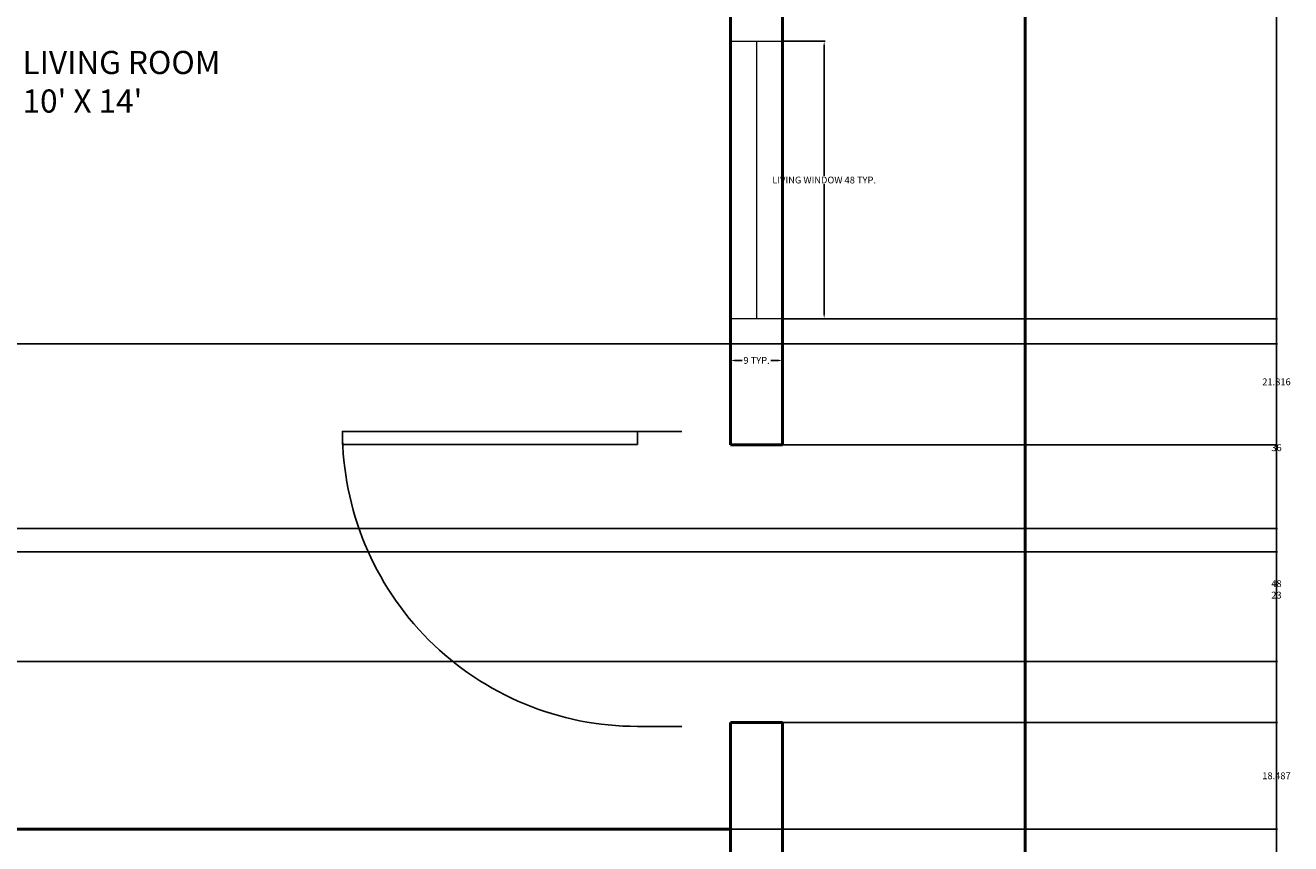
# Model space of a CAD drawing. Units: inches. Extents: x 3506 to 3958, y 1553 to 2506.
# Tile 15 of 16: x 3739 to 3958, y 2229 to 2370. Entities that reach past the tile are written whole.
import ezdxf

# ---------------------------------------------------------------- set-up
doc = ezdxf.new("R2010")
doc.units = ezdxf.units.IN
doc.header["$MEASUREMENT"] = 0
for name, color, linetype, lineweight in [('A-ANNO-DIMS', 2, 'Continuous', 18), ('A-AREA-IDEN', 7, 'Continuous', 18), ('A-WALL', 7, 'Continuous', 50), ('doors', 40, 'Continuous', 25), ('window', 30, 'Continuous', 20)]:
    doc.layers.add(name, color=color, linetype=linetype, lineweight=lineweight)
doc.layers.add('A-WALL-PATT', color=251, linetype='Continuous', lineweight=13, true_color=0x636466)
doc.styles.get("Standard").update_dxf_attribs({"font": 'arial.ttf'})
doc.dimstyles.get("Standard").update_dxf_attribs({"dimtxt": 1.18, "dimasz": 0.68, "dimexe": 0.18, "dimexo": 0.0625, "dimgap": 0.09, "dimtad": 0, "dimtih": 1, "dimtoh": 1, "dimdec": 1, "dimzin": 0, "dimdsep": 46, "dimlunit": 3, "dimtxsty": 'Standard', "dimcen": 0.09, "dimadec": 0, "dimazin": 0, "dimtfac": 1, "dimtdec": 1, "dimtofl": 0, "dimtmove": 0, "dimatfit": 3, "dimfxl": 1, "dimtolj": 1, "dimtzin": 0, "dimarcsym": 0})

# ---------------------------------------------------------------- blocks, each defined once
blk = doc.blocks.new('*U12')
for p, q in [((0, 0), (0, 6)), ((40, 0), (40, 6))]:
    blk.add_line(p, q)
blk.add_lwpolyline([(0, 0), (0, -40), (1.75, -40), (1.75, 0)], close=True)
blk.add_arc((0, 0), 40, 270, 0)
blk = doc.blocks.new('WIN-48IN-9IN-WALL')
for p, q in [((0, 48), (9, 48)), ((0, 0), (0, 48)), ((0, 48), (4.5, 48)), ((4.5, 48), (4.5, 0)), ((9, 48), (9, 0)), ((9, 0), (0, 0))]:
    blk.add_line(p, q)
blk = doc.blocks.new('*D36')
at = {"layer": 'A-ANNO-DIMS', "color": 0, "lineweight": -2, "transparency": 16777216}
for p, q in [((3869.79, 2367.7), (3877.11, 2367.7)), ((3876.93, 2367.02), (3876.93, 2344.4)), ((3876.93, 2320.38), (3876.93, 2343)), ((3869.79, 2319.7), (3877.11, 2319.7))]:
    blk.add_line(p, q, dxfattribs=at)
at = {"layer": 'A-ANNO-DIMS', "color": 0, "transparency": 16777216}
for points in [[(3876.82, 2367.02), (3877.04, 2367.02), (3876.93, 2367.7)], [(3876.82, 2320.38), (3877.04, 2320.38), (3876.93, 2319.7)]]:
    blk.add_solid(points, dxfattribs=at)
at = {"layer": 'Defpoints', "color": 0, "transparency": 16777216}
for p in [(3869.73, 2367.7), (3876.93, 2367.7), (3869.73, 2319.7)]:
    blk.add_point(p, dxfattribs=at)
at = {"layer": 'A-ANNO-DIMS', "color": 0, "transparency": 16777216, "insert": (3876.93, 2343.7), "char_height": 1.18, "attachment_point": 5}
blk.add_mtext('\\A1;LIVING WINDOW 48 TYP.', dxfattribs=at)
blk = doc.blocks.new('*D37')
at = {"layer": 'A-ANNO-DIMS', "color": 0, "lineweight": -2, "transparency": 16777216}
for p, q in [((3860.73, 2319.64), (3860.73, 2312.32)), ((3869.73, 2319.64), (3869.73, 2312.32)), ((3861.41, 2312.5), (3862.73, 2312.5)), ((3869.05, 2312.5), (3867.73, 2312.5))]:
    blk.add_line(p, q, dxfattribs=at)
at = {"layer": 'A-ANNO-DIMS', "color": 0, "transparency": 16777216}
for points in [[(3861.41, 2312.61), (3861.41, 2312.38), (3860.73, 2312.5)], [(3869.05, 2312.61), (3869.05, 2312.38), (3869.73, 2312.5)]]:
    blk.add_solid(points, dxfattribs=at)
at = {"layer": 'Defpoints', "color": 0, "transparency": 16777216}
for p in [(3860.73, 2319.7), (3869.73, 2319.7), (3869.73, 2312.5)]:
    blk.add_point(p, dxfattribs=at)
at = {"layer": 'A-ANNO-DIMS', "color": 0, "transparency": 16777216, "insert": (3865.23, 2312.5), "char_height": 1.18, "attachment_point": 5}
blk.add_mtext('\\A1;9 TYP.', dxfattribs=at)
blk = doc.blocks.new('*D39')
at = {"layer": 'A-ANNO-DIMS', "color": 0, "lineweight": -2, "transparency": 16777216}
for p, q in [((3911.79, 2461.39), (3955.36, 2461.39)), ((3955.18, 2460.71), (3955.18, 2030.09)), ((3955.18, 1598.07), (3955.18, 2028.7)), ((3911.79, 1597.39), (3955.36, 1597.39))]:
    blk.add_line(p, q, dxfattribs=at)
at = {"layer": 'A-ANNO-DIMS', "color": 0, "transparency": 16777216}
for points in [[(3955.07, 2460.71), (3955.29, 2460.71), (3955.18, 2461.39)], [(3955.07, 1598.07), (3955.29, 1598.07), (3955.18, 1597.39)]]:
    blk.add_solid(points, dxfattribs=at)
at = {"layer": 'Defpoints', "color": 0, "transparency": 16777216}
for p in [(3911.73, 2461.39), (3955.18, 2461.39), (3911.73, 1597.39)]:
    blk.add_point(p, dxfattribs=at)
at = {"layer": 'A-ANNO-DIMS', "color": 0, "transparency": 16777216, "insert": (3955.18, 2029.39), "char_height": 1.18, "attachment_point": 5}
blk.add_mtext('\\A1;864', dxfattribs=at)
blk = doc.blocks.new('*D44')
at = {"layer": 'A-ANNO-DIMS', "color": 0, "lineweight": -2, "transparency": 16777216}
for p, q in [((3911.67, 2461.39), (3508.1, 2461.39)), ((3508.28, 2460.71), (3508.28, 2344.59)), ((3508.28, 2227.07), (3508.28, 2343.2)), ((3560.67, 2226.39), (3508.1, 2226.39))]:
    blk.add_line(p, q, dxfattribs=at)
at = {"layer": 'A-ANNO-DIMS', "color": 0, "transparency": 16777216}
for points in [[(3508.17, 2460.71), (3508.39, 2460.71), (3508.28, 2461.39)], [(3508.17, 2227.07), (3508.39, 2227.07), (3508.28, 2226.39)]]:
    blk.add_solid(points, dxfattribs=at)
at = {"layer": 'Defpoints', "color": 0, "transparency": 16777216}
for p in [(3508.28, 2461.39), (3911.73, 2461.39), (3560.73, 2226.39)]:
    blk.add_point(p, dxfattribs=at)
at = {"layer": 'A-ANNO-DIMS', "color": 0, "transparency": 16777216, "insert": (3508.28, 2343.89), "char_height": 1.18, "attachment_point": 5}
blk.add_mtext('\\A1;235', dxfattribs=at)
blk = doc.blocks.new('*D48')
at = {"layer": 'A-ANNO-DIMS', "color": 0, "lineweight": -2, "transparency": 16777216}
for p, q in [((3869.79, 2297.88), (3955.36, 2297.88)), ((3955.18, 2297.2), (3955.18, 2274.57)), ((3955.18, 2250.56), (3955.18, 2273.19)), ((3869.79, 2249.88), (3955.36, 2249.88))]:
    blk.add_line(p, q, dxfattribs=at)
at = {"layer": 'A-ANNO-DIMS', "color": 0, "transparency": 16777216}
for points in [[(3955.07, 2297.2), (3955.29, 2297.2), (3955.18, 2297.88)], [(3955.07, 2250.56), (3955.29, 2250.56), (3955.18, 2249.88)]]:
    blk.add_solid(points, dxfattribs=at)
at = {"layer": 'Defpoints', "color": 0, "transparency": 16777216}
for p in [(3869.73, 2297.88), (3869.73, 2249.88), (3955.18, 2249.88)]:
    blk.add_point(p, dxfattribs=at)
at = {"layer": 'A-ANNO-DIMS', "color": 0, "transparency": 16777216, "insert": (3955.18, 2273.88), "char_height": 1.18, "attachment_point": 5}
blk.add_mtext('\\A1;48', dxfattribs=at)
blk = doc.blocks.new('*D49')
at = {"layer": 'A-ANNO-DIMS', "color": 0, "lineweight": -2, "transparency": 16777216}
for p, q in [((3869.79, 2249.88), (3955.36, 2249.88)), ((3955.18, 2249.2), (3955.18, 2241.33)), ((3955.18, 2232.07), (3955.18, 2239.95)), ((3860.79, 2231.39), (3955.36, 2231.39))]:
    blk.add_line(p, q, dxfattribs=at)
at = {"layer": 'A-ANNO-DIMS', "color": 0, "transparency": 16777216}
for points in [[(3955.07, 2249.2), (3955.29, 2249.2), (3955.18, 2249.88)], [(3955.07, 2232.07), (3955.29, 2232.07), (3955.18, 2231.39)]]:
    blk.add_solid(points, dxfattribs=at)
at = {"layer": 'Defpoints', "color": 0, "transparency": 16777216}
for p in [(3869.73, 2249.88), (3860.73, 2231.39), (3955.18, 2231.39)]:
    blk.add_point(p, dxfattribs=at)
at = {"layer": 'A-ANNO-DIMS', "color": 0, "transparency": 16777216, "insert": (3955.18, 2240.64), "char_height": 1.18, "attachment_point": 5}
blk.add_mtext('\\A1;18.487', dxfattribs=at)
blk = doc.blocks.new('*D54')
at = {"layer": 'A-ANNO-DIMS', "color": 0, "lineweight": -2, "transparency": 16777216}
for p, q in [((3869.79, 2319.7), (3955.36, 2319.7)), ((3955.18, 2319.02), (3955.18, 2309.48)), ((3955.18, 2298.56), (3955.18, 2308.1)), ((3869.79, 2297.88), (3955.36, 2297.88))]:
    blk.add_line(p, q, dxfattribs=at)
at = {"layer": 'A-ANNO-DIMS', "color": 0, "transparency": 16777216}
for points in [[(3955.07, 2319.02), (3955.29, 2319.02), (3955.18, 2319.7)], [(3955.07, 2298.56), (3955.29, 2298.56), (3955.18, 2297.88)]]:
    blk.add_solid(points, dxfattribs=at)
at = {"layer": 'Defpoints', "color": 0, "transparency": 16777216}
for p in [(3869.73, 2319.7), (3869.73, 2297.88), (3955.18, 2297.88)]:
    blk.add_point(p, dxfattribs=at)
at = {"layer": 'A-ANNO-DIMS', "color": 0, "transparency": 16777216, "insert": (3955.18, 2308.79), "char_height": 1.18, "attachment_point": 5}
blk.add_mtext('\\A1;21.816', dxfattribs=at)
blk = doc.blocks.new('*D67')
at = {"layer": 'A-ANNO-DIMS', "color": 0, "lineweight": -2, "transparency": 16777216}
for p, q in [((3697.79, 2315.39), (3955.36, 2315.39)), ((3955.18, 2314.71), (3955.18, 2298.09)), ((3955.18, 2280.07), (3955.18, 2296.7)), ((3699.79, 2279.39), (3955.36, 2279.39))]:
    blk.add_line(p, q, dxfattribs=at)
at = {"layer": 'A-ANNO-DIMS', "color": 0, "transparency": 16777216}
for points in [[(3955.07, 2314.71), (3955.29, 2314.71), (3955.18, 2315.39)], [(3955.07, 2280.07), (3955.29, 2280.07), (3955.18, 2279.39)]]:
    blk.add_solid(points, dxfattribs=at)
at = {"layer": 'Defpoints', "color": 0, "transparency": 16777216}
for p in [(3697.73, 2315.39), (3699.73, 2279.39), (3955.18, 2279.39)]:
    blk.add_point(p, dxfattribs=at)
at = {"layer": 'A-ANNO-DIMS', "color": 0, "transparency": 16777216, "insert": (3955.18, 2297.39), "char_height": 1.18, "attachment_point": 5}
blk.add_mtext('\\A1;36', dxfattribs=at)
blk = doc.blocks.new('*D69')
at = {"layer": 'A-ANNO-DIMS', "color": 0, "lineweight": -2, "transparency": 16777216}
for p, q in [((3630.79, 2283.39), (3955.36, 2283.39)), ((3955.18, 2282.71), (3955.18, 2272.59)), ((3955.18, 2261.07), (3955.18, 2271.2)), ((3630.79, 2260.39), (3955.36, 2260.39))]:
    blk.add_line(p, q, dxfattribs=at)
at = {"layer": 'A-ANNO-DIMS', "color": 0, "transparency": 16777216}
for points in [[(3955.07, 2282.71), (3955.29, 2282.71), (3955.18, 2283.39)], [(3955.07, 2261.07), (3955.29, 2261.07), (3955.18, 2260.39)]]:
    blk.add_solid(points, dxfattribs=at)
at = {"layer": 'Defpoints', "color": 0, "transparency": 16777216}
for p in [(3630.73, 2283.39), (3630.73, 2260.39), (3955.18, 2260.39)]:
    blk.add_point(p, dxfattribs=at)
at = {"layer": 'A-ANNO-DIMS', "color": 0, "transparency": 16777216, "insert": (3955.18, 2271.89), "char_height": 1.18, "attachment_point": 5}
blk.add_mtext('\\A1;23', dxfattribs=at)

msp = doc.modelspace()

# ---------------------------------------------------------------- hatches: boundary and pattern name
at = {"layer": 'A-WALL-PATT'}
h = msp.add_hatch(dxfattribs=at)
h.set_pattern_fill('ANSI31', color=256)
h.paths.add_polyline_path([(3911.7302, 2461.3942), (3551.7302, 2461.3942), (3551.7302, 2152.516), (3560.7302, 2152.516), (3560.7302, 2116.516), (3551.7302, 2116.516), (3551.7302, 1920.5711), (3556.2302, 1920.5711), (3560.7302, 1920.5711), (3560.7302, 2000.3942), (3692.7302, 2000.3942), (3692.7302, 1997.3942), (3697.7302, 1997.3942), (3697.7302, 2000.3942), (3771.7302, 2000.3942), (3771.7302, 1997.3942), (3776.7302, 1997.3942), (3776.7302, 1997.7206), (3778.5802, 1997.7206), (3807.5802, 1997.7206), (3807.5802, 1996.4519), (3778.5802, 1996.4519), (3778.5802, 1997.7206), (3776.7302, 1997.7206), (3776.7302, 1997.3942), (3771.7302, 1997.3942), (3771.7302, 2000.3942), (3697.7302, 2000.3942), (3697.7302, 1997.3942), (3692.7302, 1997.3942), (3689.8302, 1997.3942), (3689.8302, 1995.8192), (3653.8302, 1995.8192), (3653.8302, 1997.3942), (3689.8302, 1997.3942), (3692.7302, 1997.3942), (3692.7302, 2000.3942), (3560.7302, 2000.3942), (3560.7302, 1920.5711), (3551.7302, 1920.5711), (3551.7302, 1884.5711), (3551.7302, 1597.3942), (3911.7302, 1597.3942)], flags=17)
h.paths.add_polyline_path([(3596.7302, 2005.3942), (3596.7302, 2057.3035, -0.38730371), (3569.1778, 2085), (3569.15, 2085), (3569.15, 2086.2688), (3598.15, 2086.2688), (3598.15, 2085), (3569.1778, 2085, 0.38730371), (3596.7302, 2057.3035), (3596.7302, 2057.3942), (3601.7302, 2057.3942), (3601.7302, 2055.3942), (3630.7302, 2055.3942), (3630.7302, 2034.3942), (3694.7302, 2034.3942), (3694.7302, 2053.3942), (3699.7302, 2053.3942), (3699.7302, 2005.3942), (3860.7302, 2005.3942), (3860.7302, 2173.3942), (3771.7302, 2173.3942), (3771.7302, 2194.3942), (3776.7302, 2194.3942), (3776.7302, 2178.3942), (3860.7302, 2178.3942), (3860.7302, 2231.3942), (3601.7302, 2231.3942), (3601.7302, 2241.426), (3596.7302, 2241.426), (3596.7302, 2231.3942), (3560.7302, 2231.3942), (3560.7302, 2315.3942), (3596.7302, 2315.3942), (3596.7302, 2312.3942), (3601.7302, 2312.3942), (3601.7302, 2315.3942), (3697.7302, 2315.3942), (3697.7302, 2413.3942), (3692.7302, 2413.3942), (3692.7302, 2320.3942), (3560.7302, 2320.3942), (3560.7302, 2452.3942), (3692.7302, 2452.3942), (3692.7302, 2449.3942), (3697.7302, 2449.3942), (3697.7302, 2452.3942), (3771.7302, 2452.3942), (3771.7302, 2449.3942), (3776.7302, 2449.3942), (3776.7302, 2452.3942), (3860.7302, 2452.3942), (3860.7302, 2437.2075), (3865.2302, 2437.2075), (3865.2302, 2413.2075), (3860.7302, 2413.2075), (3860.7302, 2367.6976), (3865.2302, 2367.6976), (3869.7302, 2367.6976), (3869.7302, 2319.6976), (3860.7302, 2319.6976), (3860.7302, 2211.6248), (3869.7302, 2211.6248), (3869.7302, 2187.6248), (3860.7302, 2187.6248), (3860.7302, 2138.4346), (3865.2302, 2138.4346), (3869.7302, 2138.4346), (3869.7302, 2090.4346), (3860.7302, 2090.4346), (3860.7302, 1985.8449), (3869.7302, 1985.8449), (3869.7302, 1961.8449), (3860.7302, 1961.8449), (3860.7302, 1897.0756), (3865.2302, 1897.0756), (3869.7302, 1897.0756), (3869.7302, 1849.0756), (3860.7302, 1849.0756), (3860.7302, 1847.8112), (3860.7302, 1779.3942), (3596.7302, 1779.3942), (3596.7302, 1831.3942), (3601.7302, 1831.3942), (3601.7302, 1828.3942), (3630.7302, 1828.3942), (3630.7302, 1808.3942), (3691.7302, 1808.3942), (3691.7302, 1815.3942), (3696.7302, 1815.3942), (3696.7302, 1779.3942), (3860.7302, 1779.3942), (3860.7302, 1947.3942), (3771.7302, 1947.3942), (3771.7302, 1968.3942), (3776.7302, 1968.3942), (3776.7302, 1952.3942), (3860.7302, 1952.3942), (3860.7302, 2005.3942)], flags=0)
h.paths.add_polyline_path([(3596.7302, 2038.8546), (3601.7302, 2038.8546), (3601.7302, 2014.8546), (3596.7302, 2014.8546)], flags=0)
h.paths.add_polyline_path([(3564.1688, 2107), (3564.1688, 2167), (3644.1688, 2167), (3644.1688, 2107)], flags=0)
h.paths.add_polyline_path([(3607.0972, 2052.0208), (3620.8472, 2052.0208, -0.41421356), (3621.9931, 2050.875), (3621.9931, 2025.6667, -0.41421356), (3620.8472, 2024.5208), (3607.0972, 2024.5208, -0.41421356), (3605.9514, 2025.6667), (3605.9514, 2050.875, -0.41421356)], flags=0)
h.paths.add_polyline_path([(3578.5688, 2115), (3565.3688, 2115), (3565.3688, 2135.8), (3578.5688, 2135.8), (3578.5688, 2138.2), (3565.3688, 2138.2), (3565.3688, 2159), (3580.5688, 2159), (3580.5688, 2153.8), (3593.7688, 2167), (3593.7688, 2151.8), (3578.5688, 2151.8)], flags=0)
h.paths.add_polyline_path([(3610.9167, 2050.875), (3620.0833, 2050.875, -0.41421356), (3620.8472, 2050.1111), (3620.8472, 2039.6076, -0.41421356), (3620.0833, 2038.8438), (3610.9167, 2038.8438, -0.41421356), (3610.1528, 2039.6076), (3610.1528, 2050.1111, -0.41421356)], flags=0)
h.paths.add_polyline_path([(3610.9167, 2037.6979), (3620.0833, 2037.6979, -0.41421356), (3620.8472, 2036.934), (3620.8472, 2026.4306, -0.41421356), (3620.0833, 2025.6667), (3610.9167, 2025.6667, -0.41421356), (3610.1528, 2026.4306), (3610.1528, 2036.934, -0.41421356)], flags=0)
h.paths.add_polyline_path([(3616.2639, 2044.7639, -1), (3614.7361, 2044.7639, -1)], flags=0)
h.paths.add_polyline_path([(3615.8819, 2044.7639, -1), (3615.1181, 2044.7639, -1)], flags=0)
h.paths.add_polyline_path([(3616.2639, 2031.7778, -1), (3614.7361, 2031.7778, -1)], flags=0)
h.paths.add_polyline_path([(3615.8819, 2031.7778, -1), (3615.1181, 2031.7778, -1)], flags=0)
h.paths.add_polyline_path([(3609.7539, 2021.7868), (3626.9586, 2021.7868), (3626.9586, 2008.8833), (3609.7539, 2008.8833)], flags=0)
h.paths.add_polyline_path([(3610.4708, 2021.07), (3621.2237, 2021.07), (3621.2237, 2009.6002), (3610.4708, 2009.6002)], flags=0)
h.paths.add_polyline_path([(3611.5461, 2019.9947), (3620.1484, 2019.9947), (3620.1484, 2010.6755), (3611.5461, 2010.6755)], flags=0)
h.paths.add_polyline_path([(3621.9405, 2021.07), (3626.2417, 2021.07), (3626.2417, 2009.6002), (3621.9405, 2009.6002)], flags=0)
h.paths.add_polyline_path([(3622.6574, 2020.3531), (3625.5248, 2020.3531), (3625.5248, 2017.4857), (3622.6574, 2017.4857)], flags=0)
h.paths.add_polyline_path([(3622.6574, 2016.7688), (3625.5248, 2016.7688), (3625.5248, 2010.317), (3622.6574, 2010.317)], flags=0)
h.paths.add_polyline_path([(3624.808, 2016.0519), (3624.808, 2013.9013), (3624.0911, 2013.9013), (3624.0911, 2013.1845), (3623.3743, 2013.1845), (3623.3743, 2013.9013), (3623.3743, 2016.0519)], flags=0)
h.paths.add_polyline_path([(3623.0158, 2012.8261), (3625.1664, 2012.8261), (3625.1664, 2012.1092), (3623.0158, 2012.1092)], flags=0)
h.paths.add_polyline_path([(3623.0158, 2011.7508), (3625.1664, 2011.7508), (3625.1664, 2011.0339), (3623.0158, 2011.0339)], flags=0)
h.paths.add_polyline_path([(3650.0591, 2031.8202), (3674.0368, 2031.8202), (3674.0368, 2012.638), (3669.2413, 2012.638), (3669.2413, 2011.8388), (3672.4383, 2011.8388), (3672.4383, 2011.0395), (3651.6576, 2011.0395), (3651.6576, 2011.8388), (3654.8546, 2011.8388), (3654.8546, 2012.638), (3650.0591, 2012.638)], flags=0)
h.paths.add_polyline_path([(3658.0517, 2024.6269, -1), (3651.6576, 2024.6269, -1)], flags=0)
h.paths.add_polyline_path([(3657.2524, 2024.6269, -1), (3652.4569, 2024.6269, -1)], flags=0)
h.paths.add_polyline_path([(3656.4532, 2024.6269, -1), (3653.2561, 2024.6269, -1)], flags=0)
h.paths.add_polyline_path([(3655.6539, 2024.6269, -1), (3654.0554, 2024.6269, -1)], flags=0)
h.paths.add_polyline_path([(3657.2524, 2017.4336, -1), (3652.4569, 2017.4336, -1)], flags=0)
h.paths.add_polyline_path([(3656.4532, 2017.4336, -1), (3653.2561, 2017.4336, -1)], flags=0)
h.paths.add_polyline_path([(3655.6539, 2017.4336, -1), (3654.0554, 2017.4336, -1)], flags=0)
h.paths.add_polyline_path([(3659.6502, 2027.8239), (3664.4457, 2027.8239), (3664.4457, 2015.0358), (3659.6502, 2015.0358)], flags=0)
h.paths.add_polyline_path([(3663.6465, 2027.0247), (3663.6465, 2015.8351), (3660.4494, 2015.8351), (3660.4494, 2027.0247)], flags=0)
h.paths.add_polyline_path([(3562.6688, 1945.5), (3642.6688, 1945.5), (3642.6688, 1885.5), (3562.6688, 1885.5)], flags=0)
h.paths.add_polyline_path([(3671.6391, 2024.6269, -1), (3666.8435, 2024.6269, -1)], flags=0)
h.paths.add_polyline_path([(3670.8398, 2024.6269, -1), (3667.6428, 2024.6269, -1)], flags=0)
h.paths.add_polyline_path([(3672.4383, 2017.4336, -1), (3666.0443, 2017.4336, -1)], flags=0)
h.paths.add_polyline_path([(3670.0405, 2024.6269, -1), (3668.442, 2024.6269, -1)], flags=0)
h.paths.add_polyline_path([(3671.6391, 2017.4336, -1), (3666.8435, 2017.4336, -1)], flags=0)
h.paths.add_polyline_path([(3670.8398, 2017.4336, -1), (3667.6428, 2017.4336, -1)], flags=0)
h.paths.add_polyline_path([(3592.2688, 1945.5), (3592.2688, 1930.3), (3577.0688, 1930.3), (3577.0688, 1893.5), (3563.8688, 1893.5), (3563.8688, 1914.3), (3577.0688, 1914.3), (3577.0688, 1916.7), (3563.8688, 1916.7), (3563.8688, 1937.5), (3579.0688, 1937.5), (3579.0688, 1932.3)], flags=0)
h.paths.add_polyline_path([(3670.0405, 2017.4336, -1), (3668.442, 2017.4336, -1)], flags=0)
h.paths.add_polyline_path([(3596.7302, 2283.3942), (3601.7302, 2283.3942), (3601.7302, 2265.426), (3599.2302, 2265.426), (3599.2302, 2241.426), (3596.7302, 2241.426), (3596.7302, 2265.426)], flags=0)
h.paths.add_polyline_path([(3596.7302, 1810.7006), (3601.7302, 1810.7006), (3601.7302, 1786.7006), (3596.7302, 1786.7006)], flags=0)
h.paths.add_polyline_path([(3560.7302, 1770.3942), (3738.7302, 1770.3942), (3738.7302, 1746.3942), (3738.7302, 1722.3942), (3748.7302, 1722.3942), (3748.7302, 1674.3942), (3560.7302, 1674.3942)], flags=0)
h.paths.add_polyline_path([(3728.7302, 1746.3942), (3728.7302, 1756.0642), (3738.7302, 1746.3942), (3728.7302, 1738.1582), (3728.7302, 1698.3942), (3591.2519, 1698.3942), (3591.2519, 1746.3942)], flags=0)
h.paths.add_polyline_path([(3771.7302, 2399.3942), (3771.7302, 2420.3942), (3776.7302, 2420.3942), (3776.7302, 2404.3942), (3776.7302, 2399.3942)], flags=0)
h.paths.add_polyline_path([(3911.7302, 2461.3942), (3551.7302, 2461.3942), (3551.7302, 2152.516), (3560.7302, 2152.516), (3560.7302, 2116.516), (3551.7302, 2116.516), (3551.7302, 1920.5711), (3560.7302, 1920.5711), (3560.7302, 2000.3942), (3692.7302, 2000.3942), (3692.7302, 1997.3942), (3697.7302, 1997.3942), (3697.7302, 2000.3942), (3771.7302, 2000.3942), (3771.7302, 1997.3942), (3776.7302, 1997.3942), (3776.7302, 1997.7206), (3778.5802, 1997.7206), (3807.5802, 1997.7206), (3807.5802, 1996.4519), (3778.5802, 1996.4519), (3778.5802, 1997.7206), (3776.7302, 1997.7206), (3776.7302, 1997.3942), (3771.7302, 1997.3942), (3771.7302, 2000.3942), (3697.7302, 2000.3942), (3697.7302, 1997.3942), (3692.7302, 1997.3942), (3689.8302, 1997.3942), (3689.8302, 1995.8192), (3653.8302, 1995.8192), (3653.8302, 1997.3942), (3689.8302, 1997.3942), (3692.7302, 1997.3942), (3692.7302, 2000.3942), (3560.7302, 2000.3942), (3560.7302, 1920.5711), (3551.7302, 1920.5711), (3551.7302, 1597.3942), (3911.7302, 1597.3942)], flags=17)

# ---------------------------------------------------------------- linework, layer by layer
at = {"layer": 'A-WALL'}
for p, q in [((3869.7302, 2461.3942), (3869.7302, 2297.8816)), ((3860.7302, 2452.3942), (3860.7302, 2297.8816)), ((3860.7302, 2297.8816), (3869.7302, 2297.8816)), ((3869.7302, 2249.8816), (3860.7302, 2249.8816)), ((3860.7302, 2249.8816), (3860.7302, 2066.516)), ((3869.7302, 2249.8816), (3869.7302, 2066.516)), ((3601.7302, 2231.3942), (3860.7302, 2231.3942))]:
    msp.add_line(p, q, dxfattribs=at)
msp.add_lwpolyline([(3551.7302, 2461.3942), (3911.7302, 2461.3942), (3911.7302, 1597.3942), (3551.7302, 1597.3942)], close=True, dxfattribs=at)

# ---------------------------------------------------------------- block references
at = {"layer": 'doors', "xscale": 1.27563568336709, "yscale": 1.27563568336709, "zscale": 1.27563568336709, "rotation": 270}
msp.add_blockref('*U12', (3844.632, 2300.2105), dxfattribs=at)
at = {"layer": 'window'}
msp.add_blockref('WIN-48IN-9IN-WALL', (3860.73, 2319.698), dxfattribs=at)

# ---------------------------------------------------------------- texts
at = {"layer": 'A-AREA-IDEN', "insert": (3738.2651, 2366.0351), "char_height": 4, "attachment_point": 1}
msp.add_mtext_dynamic_manual_height_columns("LIVING ROOM\\P10' X 14'", width=79.631666, gutter_width=1, heights=[0], dxfattribs=at)

# ---------------------------------------------------------------- dimensions: what is measured, and where the dimension line sits
at = {"layer": 'A-ANNO-DIMS'}
for base, p1, p2, override, picture, middle in [((3508.2802, 2461.3942), (3560.7302, 2226.3942), (3911.7302, 2461.3942), {"dimdec": 0, "dimlfac": 1, "dimrnd": 0, "dimzin": 0, "dimdsep": 46, "dimlunit": 2}, '*D44', (3508.2802, 2343.8942)), ((3955.1802, 2461.3942), (3911.7302, 1597.3942), (3911.7302, 2461.3942), {"dimdec": 0, "dimlfac": 1, "dimrnd": 0, "dimzin": 0, "dimdsep": 46, "dimlunit": 2}, '*D39', (3955.1802, 2029.3942)), ((3955.1802, 2297.8816), (3869.7302, 2319.6976), (3869.7302, 2297.8816), {"dimdec": 3, "dimlfac": 1, "dimrnd": 0, "dimzin": 0, "dimdsep": 46, "dimlunit": 2}, '*D54', (3955.1802, 2308.7896)), ((3955.1802, 2279.3942), (3697.7302, 2315.3942), (3699.7302, 2279.3942), {"dimdec": 0, "dimlfac": 1, "dimrnd": 0, "dimzin": 0, "dimdsep": 46, "dimlunit": 2}, '*D67', (3955.1802, 2297.3942)), ((3955.1802, 2249.8816), (3869.7302, 2297.8816), (3869.7302, 2249.8816), {"dimdec": 0, "dimlfac": 1, "dimrnd": 0, "dimzin": 0, "dimdsep": 46, "dimlunit": 2}, '*D48', (3955.1802, 2273.8816)), ((3955.1802, 2260.3942), (3630.7302, 2283.3942), (3630.7302, 2260.3942), {"dimdec": 0, "dimlfac": 1, "dimrnd": 0, "dimzin": 0, "dimdsep": 46, "dimlunit": 2}, '*D69', (3955.1802, 2271.8942)), ((3955.1802, 2231.3942), (3869.7302, 2249.8816), (3860.7302, 2231.3942), {"dimdec": 3, "dimlfac": 1, "dimrnd": 0, "dimzin": 0, "dimdsep": 46, "dimlunit": 2}, '*D49', (3955.1802, 2240.6379))]:
    dim = msp.add_linear_dim(base=base, p1=p1, p2=p2, angle=90, dimstyle='Standard', override=override, dxfattribs=at)
    dim.commit()
    dim.dimension.update_dxf_attribs({"geometry": picture, "text_midpoint": middle})
dim = msp.add_linear_dim(base=(3876.9302, 2367.6976), p1=(3869.7302, 2319.6976), p2=(3869.7302, 2367.6976), angle=90, text='LIVING WINDOW <> TYP.', dimstyle='Standard', override={"dimdec": 0, "dimlfac": 1, "dimrnd": 0, "dimzin": 0, "dimdsep": 46, "dimlunit": 2}, dxfattribs=at)
dim.commit()
dim.dimension.update_dxf_attribs({"geometry": '*D36', "text_midpoint": (3876.9302, 2343.6976)})
dim = msp.add_linear_dim(base=(3869.7302, 2312.4976), p1=(3860.7302, 2319.6976), p2=(3869.7302, 2319.6976), text='<> TYP.', dimstyle='Standard', override={"dimdec": 0, "dimlfac": 1, "dimrnd": 0, "dimzin": 0, "dimdsep": 46, "dimlunit": 2}, dxfattribs=at)
dim.commit()
dim.dimension.update_dxf_attribs({"geometry": '*D37', "text_midpoint": (3865.2302, 2312.4976)})

doc.saveas('drawing.dxf')
